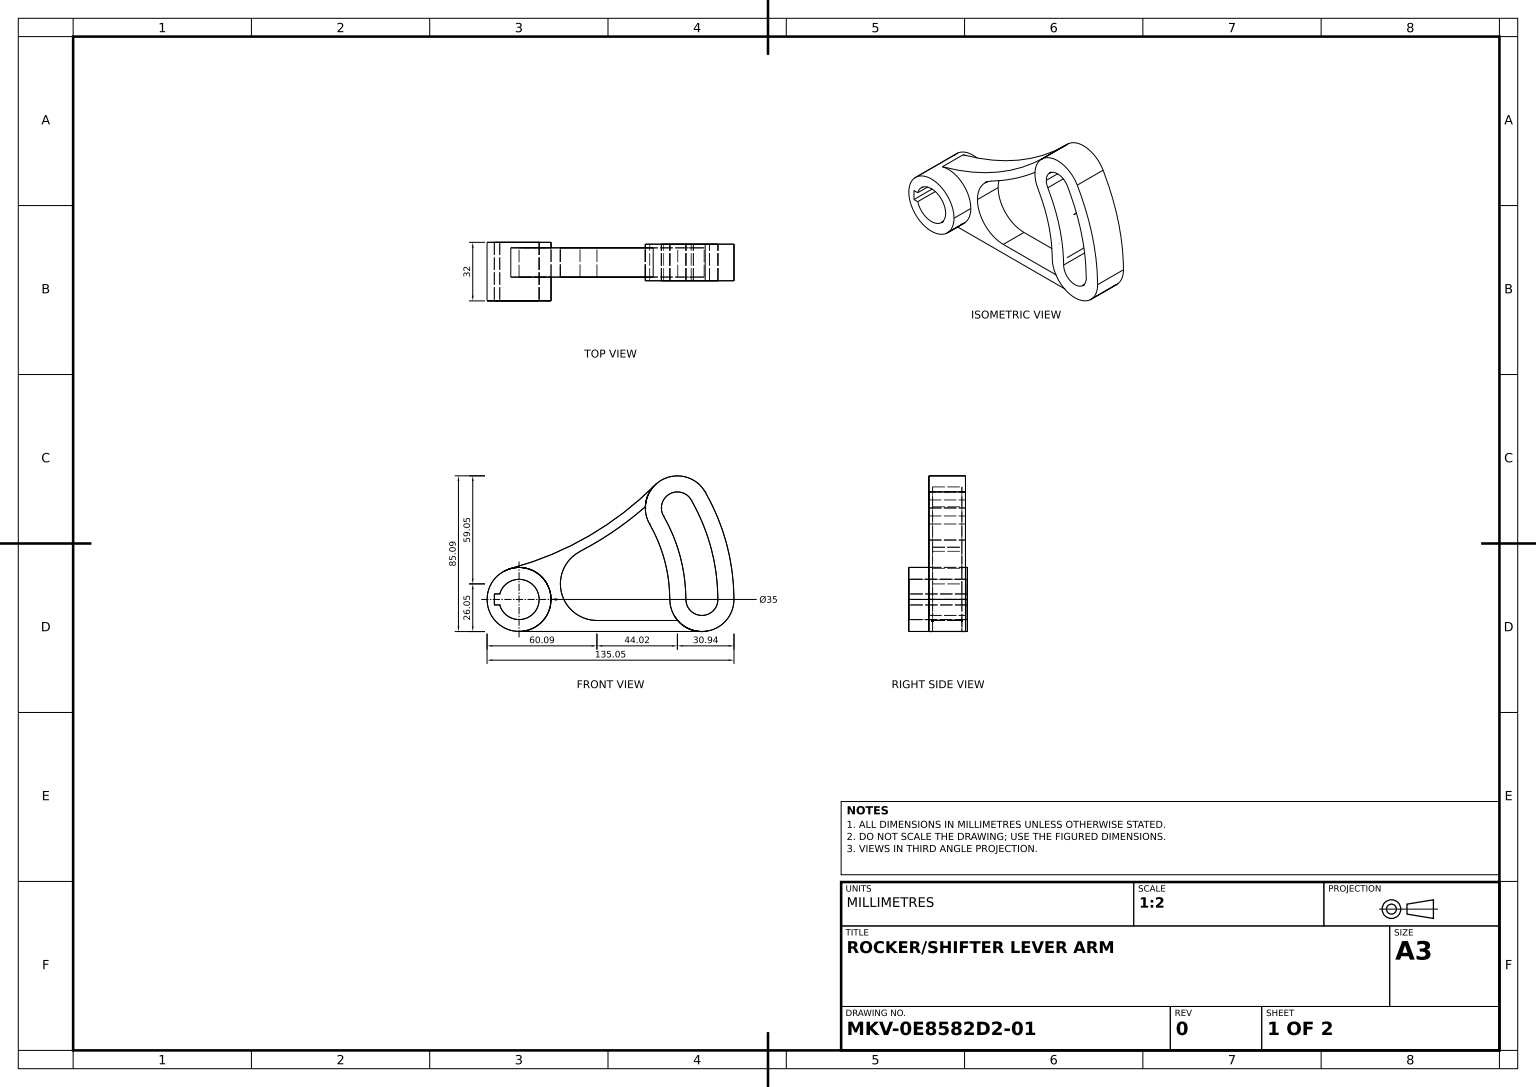
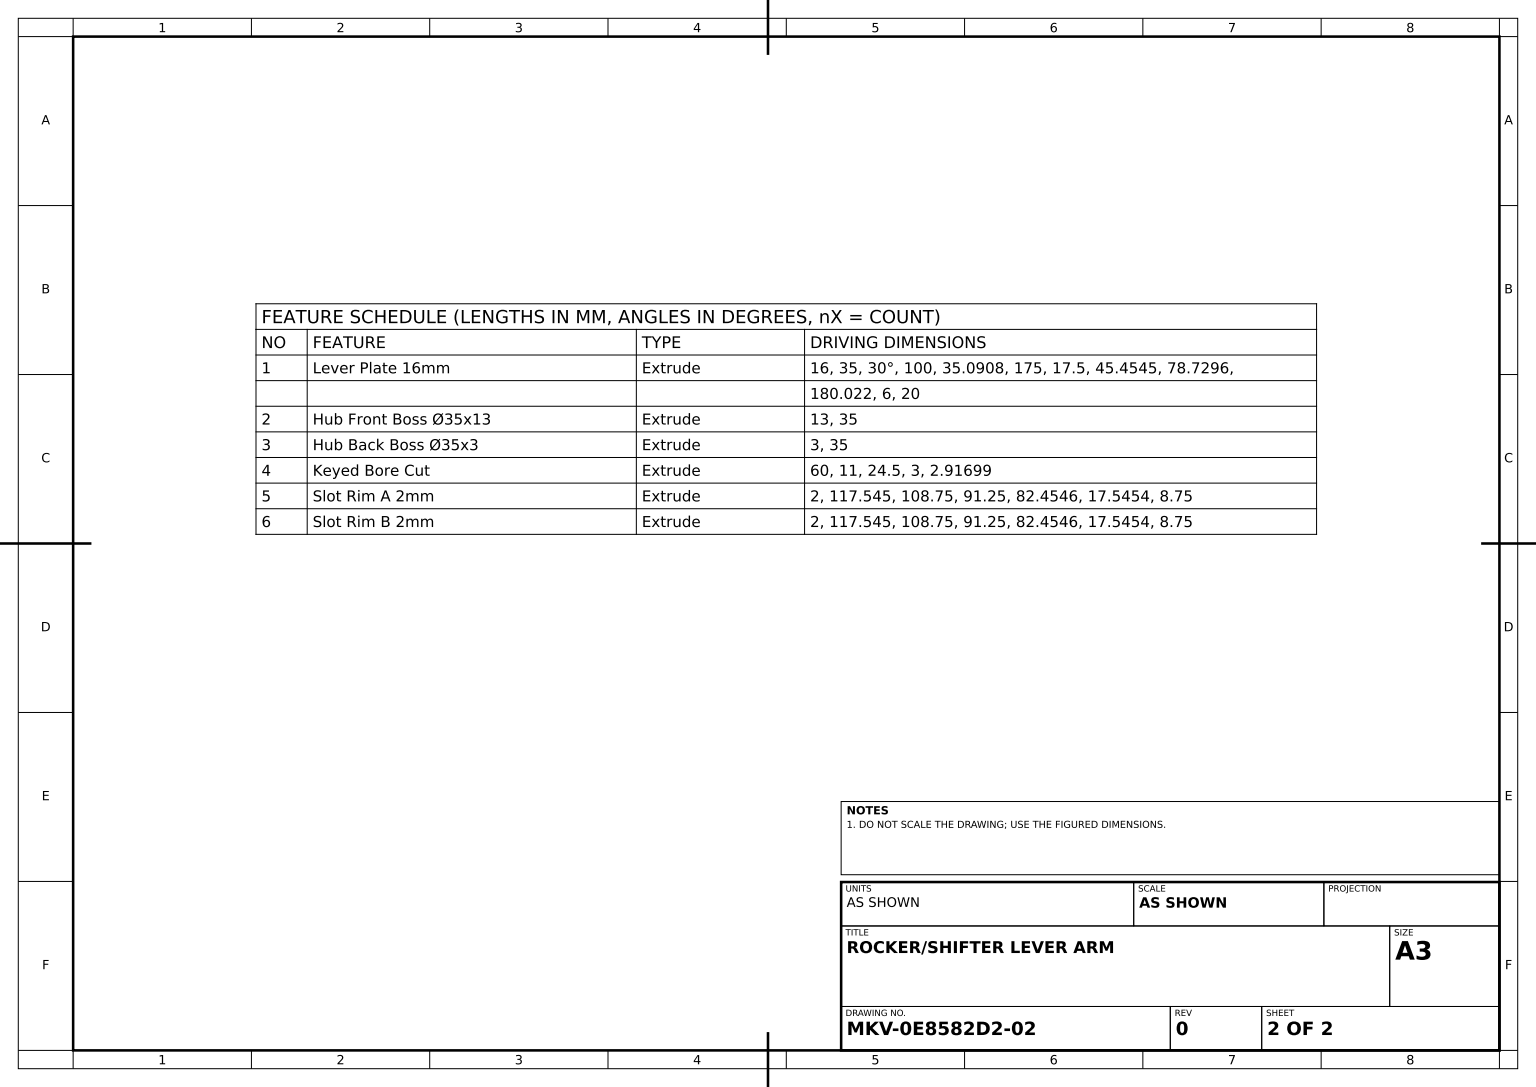
from build123d import *

# Parameters (mm, degrees)
LEVER_PLATE_16MM_DEPTH     = 16
HUB_FRONT_SKETCH_35_R      = 17.5
HUB_FRONT_BOSS_35X13_DEPTH = 13
HUB_START                  = 3
HUB_BACK_SKETCH_35_R       = 17.5
HUB_BACK_BOSS_35X3_DEPTH   = 3
KEYED_BORE_CUT_DEPTH       = 60
SLOT_RIM_A_2MM_DEPTH       = 2
SLOT_START                 = 2
SLOT_RIM_B_2MM_DEPTH       = 2


with BuildPart() as part:
    # Lever Profile Sketch → Lever Plate 16mm (new body)
    with BuildSketch(Plane.XY):
        with BuildLine():
            ThreePointArc((101.261586429, -17.5), (112.844778282, -11.952124129), (117.545415365, 0))
            ThreePointArc((117.545415365, 0), (113.540152463, 30.422992161), (101.797315804, 58.772707682))
            ThreePointArc((101.797315804, 58.772707682), (88.2863604, 67.464431009), (73.363703567, 61.514113087))
            ThreePointArc((73.363703567, 61.514113087), (37.333335855, 34.13389002), (-4.513207912, 16.9080145))
            ThreePointArc((-4.513207912, 16.9080145), (-17.351372478, -2.275933462), (0, -17.5))
            Line((0, -17.5), (101.261586429, -17.5))
        make_face()
        with BuildLine():
            ThreePointArc((71.407764953, 41.227292318), (79.645012795, 21.34081686), (82.454584635, 0))
            ThreePointArc((82.454584635, 0), (83.56318735, -6.137816406), (86.74890192, -11.5))
            Line((86.74890192, -11.5), (42.586205582, -11.5))
            ThreePointArc((42.586205582, -11.5), (23.157647429, 3.753303456), (33.364058597, 26.246887192))
            ThreePointArc((33.364058597, 26.246887192), (51.952476434, 37.375508628), (69.069413247, 50.656546497))
            ThreePointArc((69.069413247, 50.656546497), (69.572959936, 45.776850669), (71.407764953, 41.227292318))
        make_face(mode=Mode.SUBTRACT)
        with BuildLine():
            ThreePointArc((91.25, 0), (88.140731649, 23.617237866), (79.024818095, 45.625))
            ThreePointArc((79.024818095, 45.625), (82.227540378, 57.577722283), (94.180262662, 54.375))
            ThreePointArc((94.180262662, 54.375), (105.044433609, 28.146571155), (108.75, 0))
            ThreePointArc((108.75, 0), (100, -8.75), (91.25, 0))
        make_face(mode=Mode.SUBTRACT)
    extrude(amount=LEVER_PLATE_16MM_DEPTH)

    # Hub Front Sketch Ø35 → Hub Front Boss Ø35x13 (add)
    with BuildSketch(Plane.XY.offset(16)):
        with Locations(Location((0, 0, 0), (0, 0, 104.94534936))):
            Circle(HUB_FRONT_SKETCH_35_R)
    extrude(amount=HUB_FRONT_BOSS_35X13_DEPTH)

    # Hub Back Sketch Ø35 → Hub Back Boss Ø35x3 (add)
    with BuildSketch(Plane(origin=(0, 0, 0), x_dir=(-1, 0, 0), z_dir=(0, 0, -1)).offset(HUB_START)):
        Circle(HUB_BACK_SKETCH_35_R)
    extrude(amount=-HUB_BACK_BOSS_35X3_DEPTH)

    # Keyed Bore Sketch → Keyed Bore Cut (cut)
    with BuildSketch(Plane.XY.offset(29)):
        with BuildLine():
            ThreePointArc((-10.583005244, -3), (1.514421063, -10.895252583), (11, 0))
            Line((11, 0), (-13.5, 0))
            Line((-13.5, 0), (-13.5, -3))
            Line((-13.5, -3), (-10.583005244, -3))
        make_face()
        with BuildLine():
            Line((-13.5, 0), (11, 0))
            ThreePointArc((11, 0), (1.514421063, 10.895252583), (-10.583005244, 3))
            Line((-10.583005244, 3), (-13.5, 3))
            Line((-13.5, 3), (-13.5, 0))
        make_face()
    extrude(amount=-KEYED_BORE_CUT_DEPTH, mode=Mode.SUBTRACT)

    # Slot Rim Sketch A → Slot Rim A 2mm (add)
    with BuildSketch(Plane.XY.offset(16)):
        with BuildLine():
            ThreePointArc((117.545415365, 0), (113.540152463, 30.422992161), (101.797315804, 58.772707682))
            ThreePointArc((101.797315804, 58.772707682), (77.829832696, 65.194775426), (71.407764953, 41.227292318))
            ThreePointArc((71.407764953, 41.227292318), (79.645012795, 21.34081686), (82.454584635, 0))
            ThreePointArc((82.454584635, 0), (100, -17.545415365), (117.545415365, 0))
        make_face()
        with BuildLine():
            ThreePointArc((108.75, 0), (105.044433609, 28.146571155), (94.180262662, 54.375))
            ThreePointArc((94.180262662, 54.375), (82.227540378, 57.577722283), (79.024818095, 45.625))
            ThreePointArc((79.024818095, 45.625), (88.140731649, 23.617237866), (91.25, 0))
            ThreePointArc((91.25, 0), (100, -8.75), (108.75, 0))
        make_face(mode=Mode.SUBTRACT)
    extrude(amount=SLOT_RIM_A_2MM_DEPTH)

    # Slot Rim Sketch B → Slot Rim B 2mm (add)
    with BuildSketch(Plane(origin=(0, 0, 0), x_dir=(-1, 0, 0), z_dir=(0, 0, -1)).offset(SLOT_START)):
        with BuildLine():
            ThreePointArc((-101.797315804, 58.772707682), (-113.540152463, 30.422992161), (-117.545415365, 0))
            ThreePointArc((-117.545415365, 0), (-100, -17.545415365), (-82.454584635, 0))
            ThreePointArc((-82.454584635, 0), (-79.645012795, 21.34081686), (-71.407764953, 41.227292318))
            ThreePointArc((-71.407764953, 41.227292318), (-77.829832696, 65.194775426), (-101.797315804, 58.772707682))
        make_face()
        with BuildLine():
            ThreePointArc((-94.180262662, 54.375), (-105.044433609, 28.146571155), (-108.75, 0))
            ThreePointArc((-108.75, 0), (-100, -8.75), (-91.25, 0))
            ThreePointArc((-91.25, 0), (-88.140731649, 23.617237866), (-79.024818095, 45.625))
            ThreePointArc((-79.024818095, 45.625), (-82.227540378, 57.577722283), (-94.180262662, 54.375))
        make_face(mode=Mode.SUBTRACT)
    extrude(amount=-SLOT_RIM_B_2MM_DEPTH)


solid = part.part
